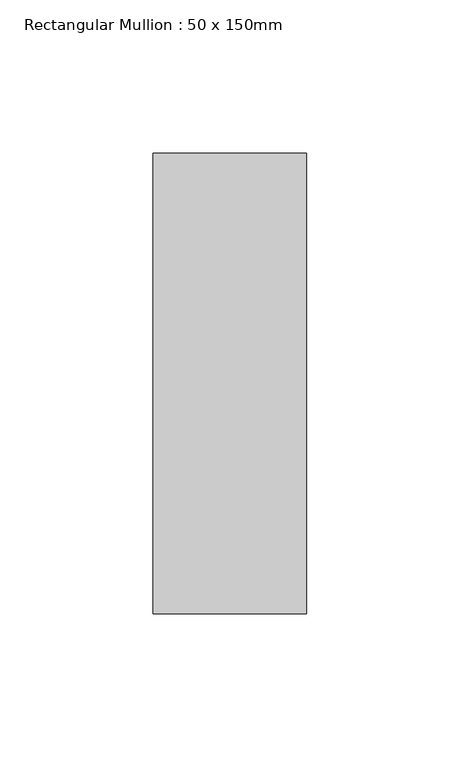
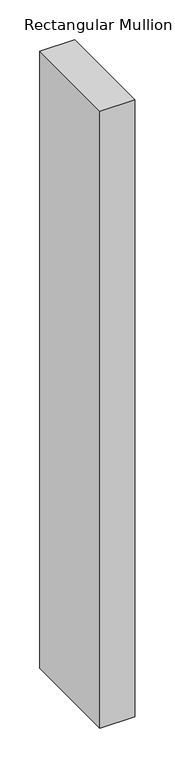
"""IFC4 building model written with IfcOpenShell, lengths in millimetres: member geometry, Rectangular Mullion : 50 x 150mm."""

from ifc_helpers import new_model, si_unit, frame, origin, place, context, project, spatial, polyline, outline, extrude, source, transform, mapped, element, save


def rectangular_mullion_50_x_150mm_e6be0bb7(model_context):
    return source(origin(), model_context, "Body", "SweptSolid", [
        extrude(outline(polyline([(0.0, 75.0), (0.0, -75.0), (-50.0, -75.0), (-50.0, 75.0), (0.0, 75.0)])), frame((0.0, 0.0, -941.6666667), z_axis=(0.0, 0.0, 1.0), x_axis=(1.0, 0.0, 0.0)), (0.0, 0.0, 1.0), 941.6666667),
    ])


if __name__ == "__main__":
    model = new_model("IFC4")
    model_context = context("Model", 3, world=origin())
    ifc_project = project(units=[si_unit("LENGTHUNIT", "METRE", prefix="MILLI")], contexts=[model_context])
    site = spatial("IfcSite", under=ifc_project)
    building = spatial("IfcBuilding", under=site)
    placement = place(None, origin())
    rectangular_mullion_50_x_150mm_shape = rectangular_mullion_50_x_150mm_e6be0bb7(model_context)
    element("IfcMember", 1, ObjectType="Rectangular Mullion : 50 x 150mm", at=placement, inside=building, context=model_context, shape_type="MappedRepresentation", body=[
        mapped(rectangular_mullion_50_x_150mm_shape, transform((0.0, 0.0, 0.0), x_axis=(1.0, 0.0, 0.0), y_axis=(0.0, 1.0, 0.0), z_axis=(0.0, 0.0, 1.0))),
    ])
    save(model, "model.ifc")

# Revit data of these elements
# Type "Rectangular Mullion : 50 x 150mm"
#   built-in parameter 1007304 = 0.492126 (stored number, unit not read)
#   built-in parameter 1007301 = 0.082021 (stored number, unit not read)
#   built-in parameter 1007300 = 0.082021 (stored number, unit not read)
# Element 1 (IfcMember, "Rectangular Mullion : 50 x 150mm")
#   Materials on its faces: "Aluminium"
# Materials
#   "Aluminium": class "Metal", colour RGB 247 247 247, transparency 0, Description = "Aluminium 6061", Cost = 0
